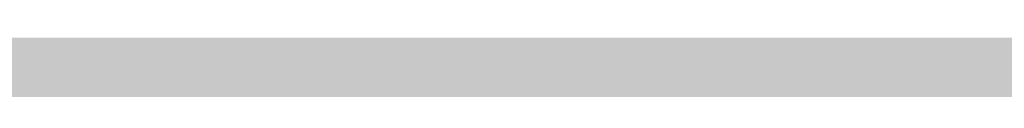
# Model space of a CAD drawing. Units: feet. Extents: x 3168 to 4724, y 827 to 1477.
# Tile 9 of 256: x 3244.72 to 3257.5, y 1098.34 to 1099. Entities that reach past the tile are written whole.
import ezdxf

# ---------------------------------------------------------------- set-up
doc = ezdxf.new("R2010")
doc.units = ezdxf.units.FT
doc.layers.add('A-ELEV', color=7, linetype='Continuous', lineweight=35)
doc.layers.add('A-ELEV-PATT', color=8, linetype='Continuous', lineweight=13)

msp = doc.modelspace()

# ---------------------------------------------------------------- hatches: boundary and pattern name
at = {"layer": 'A-ELEV-PATT'}
h = msp.add_hatch(color=256, dxfattribs=at)
h.dxf.hatch_style = 1
h.paths.add_polyline_path([(3384.525, 1099.016), (3335.029, 1099.016), (3299.317, 1099.016), (3273.143, 1099.016), (3217.565, 1099.016), (3168.069, 827.116), (3335.029, 827.116)])

# ---------------------------------------------------------------- linework, layer by layer
at = {"layer": 'A-ELEV'}
msp.add_open_spline([(3808.52, 1099.016), (3808.52, 1141.413), (3808.52, 1183.81), (3808.52, 1226.635), (3808.52, 1227.064), (3808.52, 1227.492), (3811.492, 1248.995), (3814.464, 1270.498), (3817.465, 1292.218), (3817.495, 1292.435), (3817.525, 1292.652), (3817.573, 1310.107), (3817.62, 1327.562), (3817.668, 1345.016), (3817.668, 1345.458), (3817.668, 1345.9), (3817.668, 1346.456), (3817.668, 1346.571), (3817.668, 1346.753), (3817.668, 1346.82), (3817.668, 1346.935), (3817.668, 1346.982), (3817.668, 1347.039), (3817.668, 1347.047), (3817.668, 1347.074), (3817.668, 1347.059), (3817.668, 1347.062), (3817.668, 1347.063), (3817.668, 1347.066), (3817.668, 1347.068), (3817.668, 1347.075), (3817.668, 1347.079), (3817.668, 1347.093), (3817.668, 1347.102), (3817.668, 1347.129), (3817.668, 1347.147), (3817.667, 1347.2), (3817.667, 1347.236), (3817.666, 1347.343), (3817.665, 1347.415), (3817.661, 1347.628), (3817.657, 1347.77), (3817.64, 1348.192), (3817.624, 1348.472), (3817.559, 1349.3), (3817.496, 1349.841), (3817.255, 1351.424), (3817.026, 1352.429), (3816.307, 1354.889), (3815.744, 1356.269), (3814.464, 1358.819), (3813.746, 1359.991), (3812.196, 1362.172), (3811.362, 1363.182), (3809.589, 1365.069), (3808.649, 1365.946), (3806.654, 1367.58), (3805.6, 1368.336), (3803.353, 1369.722), (3802.161, 1370.352), (3799.601, 1371.454), (3798.233, 1371.925), (3795.28, 1372.635), (3793.693, 1372.872), (3791.869, 1372.926), (3791.741, 1372.929), (3791.353, 1372.934), (3791.093, 1372.933), (3790.304, 1372.915), (3789.77, 1372.884), (3789.209, 1372.83), (3789.191, 1372.828), (3789.135, 1372.823), (3789.098, 1372.819), (3789.048, 1372.814), (3789.036, 1372.813), (3789, 1372.809), (3788.976, 1372.806), (3788.949, 1372.803), (3788.947, 1372.803), (3788.943, 1372.803), (3788.941, 1372.802), (3788.939, 1372.802), (3788.938, 1372.802), (3788.935, 1372.802), (3788.868, 1372.794), (3788.757, 1372.782), (3788.702, 1372.776), (3788.536, 1372.758), (3788.425, 1372.746), (3788.093, 1372.709), (3787.872, 1372.685), (3787.208, 1372.612), (3786.765, 1372.563), (3785.437, 1372.417), (3784.551, 1372.32), (3781.895, 1372.027), (3780.125, 1371.833), (3774.813, 1371.248), (3771.271, 1370.859), (3760.647, 1369.69), (3753.564, 1368.911), (3732.316, 1366.573), (3718.15, 1365.015), (3694.007, 1362.359), (3684.029, 1361.262), (3674.051, 1360.164), (3664.601, 1360.164), (3655.151, 1360.164), (3626.801, 1360.164), (3607.901, 1360.164), (3551.202, 1360.164), (3513.402, 1360.164), (3467.725, 1360.164), (3459.848, 1360.164), (3436.215, 1360.164), (3420.46, 1360.164), (3373.194, 1360.164), (3341.684, 1360.164), (3302.848, 1360.164), (3295.523, 1360.164), (3286.038, 1360.164), (3283.879, 1360.164), (3277.403, 1360.164), (3273.085, 1360.164), (3267.733, 1360.164), (3266.699, 1360.164), (3263.597, 1360.164), (3261.528, 1360.164), (3259.237, 1360.164), (3259.014, 1360.164), (3258.344, 1360.164), (3257.897, 1360.164), (3257.431, 1360.164), (3257.411, 1360.164), (3257.371, 1360.164), (3257.375, 1360.164), (3257.375, 1360.164), (3257.374, 1360.164), (3257.372, 1360.164), (3257.371, 1360.164), (3257.367, 1360.164), (3257.364, 1360.164), (3257.356, 1360.164), (3257.351, 1360.164), (3257.335, 1360.164), (3257.324, 1360.164), (3257.293, 1360.164), (3257.272, 1360.164), (3257.208, 1360.163), (3257.166, 1360.163), (3257.04, 1360.161), (3256.956, 1360.16), (3256.706, 1360.153), (3256.539, 1360.147), (3256.044, 1360.122), (3255.717, 1360.097), (3254.752, 1360), (3254.128, 1359.907), (3252.18, 1359.525), (3250.942, 1359.144), (3248.67, 1358.243), (3247.636, 1357.724), (3245.733, 1356.603), (3244.863, 1356.002), (3243.253, 1354.743), (3242.512, 1354.085), (3240.751, 1352.345), (3239.801, 1351.23), (3238.088, 1348.872), (3237.325, 1347.63), (3235.983, 1344.972), (3235.402, 1343.555), (3234.591, 1340.815), (3234.311, 1339.544), (3233.976, 1336.803), (3233.922, 1335.331), (3234.149, 1332.591), (3234.35, 1331.367), (3234.72, 1329.999), (3234.752, 1329.883), (3234.854, 1329.535), (3234.926, 1329.302), (3235.025, 1329.003), (3235.047, 1328.937), (3235.078, 1328.847), (3235.086, 1328.823), (3235.111, 1328.751), (3235.128, 1328.703), (3235.148, 1328.646), (3235.151, 1328.638), (3235.156, 1328.624), (3235.158, 1328.618), (3235.16, 1328.612), (3235.166, 1328.597), (3235.18, 1328.556), (3235.19, 1328.528), (3235.221, 1328.443), (3235.241, 1328.386), (3235.302, 1328.216), (3235.343, 1328.102), (3235.465, 1327.762), (3235.546, 1327.535), (3235.79, 1326.853), (3235.953, 1326.399), (3236.44, 1325.037), (3236.766, 1324.128), (3237.741, 1321.403), (3238.392, 1319.587), (3240.344, 1314.137), (3241.645, 1310.504), (3245.548, 1299.604), (3248.15, 1292.337), (3255.956, 1270.537), (3261.16, 1256.004), (3267.388, 1238.612), (3268.411, 1235.753), (3269.51, 1232.684), (3269.586, 1232.474), (3269.707, 1232.136), (3269.752, 1232.008), (3269.827, 1231.799), (3269.856, 1231.718), (3269.906, 1231.578), (3269.927, 1231.52), (3269.972, 1231.393), (3269.997, 1231.325), (3270.027, 1231.243), (3270.032, 1231.228), (3270.04, 1231.204), (3270.039, 1231.207), (3270.039, 1231.207), (3270.039, 1231.206), (3270.04, 1231.206), (3270.04, 1231.205), (3270.04, 1231.204), (3270.04, 1231.204), (3270.041, 1231.201), (3270.042, 1231.2), (3270.043, 1231.195), (3270.045, 1231.192), (3270.048, 1231.183), (3270.05, 1231.177), (3270.056, 1231.159), (3270.061, 1231.147), (3270.074, 1231.111), (3270.083, 1231.087), (3270.109, 1231.014), (3270.127, 1230.966), (3270.18, 1230.822), (3270.216, 1230.727), (3270.325, 1230.442), (3270.4, 1230.253), (3270.629, 1229.691), (3270.789, 1229.324), (3271.286, 1228.238), (3271.643, 1227.54), (3272.776, 1225.515), (3273.614, 1224.261), (3275.416, 1221.918), (3276.38, 1220.829), (3278.897, 1218.318), (3280.512, 1216.98), (3283.951, 1214.603), (3285.776, 1213.564), (3289.654, 1211.813), (3291.707, 1211.101), (3294.03, 1210.574), (3294.169, 1210.543), (3294.588, 1210.454), (3294.869, 1210.399), (3295.718, 1210.243), (3296.293, 1210.155), (3296.979, 1210.07), (3297.083, 1210.058), (3297.393, 1210.023), (3297.602, 1210.002), (3298.229, 1209.946), (3298.652, 1209.917), (3299.13, 1209.895), (3299.181, 1209.893), (3299.334, 1209.887), (3299.437, 1209.883), (3299.745, 1209.874), (3299.951, 1209.871), (3300.195, 1209.869), (3300.232, 1209.869), (3300.28, 1209.869), (3300.291, 1209.869), (3300.306, 1209.869), (3300.311, 1209.869), (3300.321, 1209.869), (3300.326, 1209.869), (3300.332, 1209.869), (3300.334, 1209.869), (3300.337, 1209.869), (3300.338, 1209.869), (3300.341, 1209.869), (3300.343, 1209.869), (3300.346, 1209.869), (3300.346, 1209.869), (3300.346, 1209.869), (3300.366, 1209.869), (3300.388, 1209.869), (3300.399, 1209.869), (3300.431, 1209.869), (3300.453, 1209.869), (3300.517, 1209.869), (3300.561, 1209.869), (3300.69, 1209.869), (3300.777, 1209.869), (3301.036, 1209.869), (3301.209, 1209.869), (3301.727, 1209.869), (3302.073, 1209.869), (3303.11, 1209.869), (3303.801, 1209.869), (3305.875, 1209.869), (3307.257, 1209.869), (3311.405, 1209.869), (3314.17, 1209.869), (3322.466, 1209.869), (3327.996, 1209.869), (3344.586, 1209.869), (3355.647, 1209.869), (3388.828, 1209.869), (3410.949, 1209.869), (3477.312, 1209.869), (3521.554, 1209.869), (3566.836, 1209.869), (3567.877, 1209.869), (3570.999, 1209.869), (3573.08, 1209.869), (3575.781, 1209.869), (3576.401, 1209.869), (3577.296, 1209.869), (3577.571, 1209.869), (3578.397, 1209.869), (3578.948, 1209.869), (3579.756, 1209.869), (3580.015, 1209.869), (3580.343, 1209.869), (3580.327, 1209.869), (3580.327, 1209.869), (3580.327, 1209.869), (3580.328, 1209.869), (3580.328, 1209.869), (3580.329, 1209.869), (3580.33, 1209.869), (3580.331, 1209.869), (3580.333, 1209.869), (3580.336, 1209.869), (3580.339, 1209.869), (3580.346, 1209.869), (3580.351, 1209.869), (3580.366, 1209.869), (3580.375, 1209.869), (3580.405, 1209.868), (3580.424, 1209.868), (3580.483, 1209.868), (3580.522, 1209.868), (3580.64, 1209.867), (3580.719, 1209.865), (3580.956, 1209.861), (3581.115, 1209.856), (3581.594, 1209.837), (3581.916, 1209.818), (3582.89, 1209.742), (3583.548, 1209.666), (3585.532, 1209.361), (3586.867, 1209.054), (3589.472, 1208.252), (3590.74, 1207.758), (3591.995, 1207.159), (3592.058, 1207.129), (3592.244, 1207.038), (3592.368, 1206.977), (3592.735, 1206.79), (3592.977, 1206.663), (3593.245, 1206.516), (3593.275, 1206.5), (3593.365, 1206.45), (3593.425, 1206.416), (3593.604, 1206.315), (3593.723, 1206.247), (3593.857, 1206.168), (3593.874, 1206.158), (3593.926, 1206.128), (3593.96, 1206.108), (3594.062, 1206.047), (3594.13, 1206.006), (3594.208, 1205.958), (3594.22, 1205.951), (3594.253, 1205.931), (3594.276, 1205.917), (3594.343, 1205.876), (3594.388, 1205.848), (3594.434, 1205.819), (3594.435, 1205.818), (3594.44, 1205.815), (3594.443, 1205.813), (3594.447, 1205.811), (3594.448, 1205.81), (3594.449, 1205.81), (3594.449, 1205.809), (3594.45, 1205.809), (3594.45, 1205.808), (3594.451, 1205.808), (3594.467, 1205.798), (3594.493, 1205.782), (3594.506, 1205.774), (3594.545, 1205.749), (3594.571, 1205.733), (3594.648, 1205.684), (3594.7, 1205.652), (3594.855, 1205.555), (3594.959, 1205.49), (3595.269, 1205.295), (3595.476, 1205.166), (3596.097, 1204.776), (3596.511, 1204.517), (3597.753, 1203.739), (3598.581, 1203.22), (3601.064, 1201.664), (3602.72, 1200.626), (3607.687, 1197.513), (3610.998, 1195.438), (3620.932, 1189.212), (3627.555, 1185.061), (3647.423, 1172.61), (3660.668, 1164.309), (3700.403, 1139.405), (3726.894, 1122.803), (3757.206, 1103.806), (3761.027, 1101.411), (3764.848, 1099.016), (3745.328, 1099.016), (3725.808, 1099.016), (3706.288, 1099.016), (3706.288, 1108.453), (3706.288, 1117.89), (3706.288, 1127.327), (3710.751, 1127.327), (3715.213, 1127.327), (3719.676, 1127.327)], degree=3, knots=[0, 0, 0, 0, 0.982037, 0.982037, 0.991957, 0.991957, 0.991957, 1.966522, 1.966522, 1.976367, 1.976367, 1.976367, 2.976367, 2.976367, 2.976367, 3.00169, 3.00169, 3.008272, 3.008272, 3.012129, 3.012129, 3.014851, 3.014851, 3.015353, 3.015353, 3.016359, 3.016359, 3.017365, 3.017365, 3.019376, 3.019376, 3.023398, 3.023398, 3.031442, 3.031442, 3.047531, 3.047531, 3.079708, 3.079708, 3.144063, 3.144063, 3.272772, 3.272772, 3.53019, 3.53019, 4.045026, 4.045026, 5.074698, 5.074698, 6.700878, 6.700878, 8.327058, 8.327058, 9.953238, 9.953238, 11.579418, 11.579418, 13.205598, 13.205598, 14.831778, 14.831778, 16.457958, 16.457958, 18.084138, 18.084138, 18.206872, 18.206872, 18.45234, 18.45234, 18.943275, 18.943275, 18.960093, 18.960093, 18.993729, 18.993729, 19.00461, 19.00461, 19.026374, 19.026374, 19.028737, 19.028737, 19.03018, 19.03018, 19.030897, 19.030897, 19.032332, 19.032332, 19.033766, 19.033766, 19.036636, 19.036636, 19.042374, 19.042374, 19.053851, 19.053851, 19.076805, 19.076805, 19.122714, 19.122714, 19.21453, 19.21453, 19.398163, 19.398163, 19.765429, 19.765429, 20.024128, 20.024128, 20.024128, 20.092031, 20.092031, 20.227836, 20.227836, 20.499446, 20.499446, 20.556051, 20.556051, 20.66926, 20.66926, 20.895678, 20.895678, 20.948316, 20.948316, 20.963829, 20.963829, 20.994855, 20.994855, 21.002285, 21.002285, 21.017146, 21.017146, 21.01875, 21.01875, 21.021959, 21.021959, 21.022102, 21.022102, 21.022249, 21.022249, 21.022708, 21.022708, 21.023627, 21.023627, 21.025464, 21.025464, 21.029138, 21.029138, 21.036486, 21.036486, 21.051183, 21.051183, 21.080575, 21.080575, 21.139361, 21.139361, 21.256932, 21.256932, 21.492073, 21.492073, 21.962356, 21.962356, 23.01002, 23.01002, 24.057684, 24.057684, 25.105348, 25.105348, 26.153011, 26.153011, 27.776787, 27.776787, 29.400562, 29.400562, 31.024337, 31.024337, 32.278801, 32.278801, 33.533265, 33.533265, 34.467568, 34.467568, 34.553971, 34.553971, 34.726776, 34.726776, 34.775309, 34.775309, 34.793079, 34.793079, 34.82862, 34.82862, 34.834979, 34.834979, 34.839039, 34.839039, 34.839411, 34.839411, 34.840285, 34.840285, 34.842034, 34.842034, 34.845531, 34.845531, 34.852525, 34.852525, 34.866512, 34.866512, 34.894488, 34.894488, 34.950439, 34.950439, 35.062342, 35.062342, 35.286147, 35.286147, 35.733758, 35.733758, 35.821815, 35.821815, 35.828283, 35.828283, 35.832225, 35.832225, 35.834724, 35.834724, 35.836521, 35.836521, 35.838617, 35.838617, 35.839073, 35.839073, 35.839345, 35.839345, 35.839617, 35.839617, 35.840161, 35.840161, 35.841249, 35.841249, 35.843425, 35.843425, 35.847778, 35.847778, 35.856482, 35.856482, 35.873891, 35.873891, 35.908709, 35.908709, 35.978345, 35.978345, 36.117617, 36.117617, 36.396161, 36.396161, 36.953248, 36.953248, 38.067423, 38.067423, 40.295772, 40.295772, 42.524122, 42.524122, 45.81453, 45.81453, 49.104937, 49.104937, 52.395345, 52.395345, 52.603776, 52.603776, 53.020639, 53.020639, 53.854363, 53.854363, 54.001655, 54.001655, 54.296238, 54.296238, 54.885405, 54.885405, 54.955785, 54.955785, 55.096546, 55.096546, 55.378067, 55.378067, 55.42849, 55.42849, 55.442691, 55.442691, 55.449436, 55.449436, 55.455957, 55.455957, 55.458409, 55.458409, 55.459872, 55.459872, 55.462798, 55.462798, 55.462856, 55.462856, 55.462972, 55.462972, 55.463088, 55.463088, 55.463319, 55.463319, 55.463782, 55.463782, 55.464708, 55.464708, 55.46656, 55.46656, 55.470263, 55.470263, 55.47767, 55.47767, 55.492484, 55.492484, 55.522112, 55.522112, 55.581369, 55.581369, 55.699882, 55.699882, 55.936907, 55.936907, 56.410959, 56.410959, 56.42211, 56.42211, 56.444413, 56.444413, 56.451051, 56.451051, 56.454001, 56.454001, 56.459901, 56.459901, 56.462666, 56.462666, 56.463418, 56.463418, 56.464171, 56.464171, 56.465675, 56.465675, 56.468684, 56.468684, 56.474702, 56.474702, 56.486738, 56.486738, 56.51081, 56.51081, 56.558955, 56.558955, 56.655243, 56.655243, 56.847821, 56.847821, 57.232975, 57.232975, 58.003284, 58.003284, 59.543901, 59.543901, 62.625137, 62.625137, 68.787607, 68.787607, 74.950078, 74.950078, 75.27336, 75.27336, 75.919923, 75.919923, 77.213051, 77.213051, 77.377769, 77.377769, 77.707206, 77.707206, 78.366079, 78.366079, 78.462532, 78.462532, 78.655436, 78.655436, 79.041245, 79.041245, 79.105735, 79.105735, 79.234714, 79.234714, 79.492672, 79.492672, 79.502197, 79.502197, 79.521249, 79.521249, 79.523534, 79.523534, 79.528103, 79.528103, 79.528682, 79.528682, 79.528885, 79.528885, 79.529089, 79.529089, 79.529495, 79.529495, 79.530308, 79.530308, 79.531935, 79.531935, 79.535187, 79.535187, 79.541693, 79.541693, 79.554704, 79.554704, 79.580725, 79.580725, 79.632769, 79.632769, 79.736856, 79.736856, 79.94503, 79.94503, 80.361377, 80.361377, 80.421435, 80.421435, 80.421435, 81.421435, 81.421435, 81.421435, 82.421435, 82.421435, 82.421435, 83.421435, 83.421435, 83.421435, 83.421435], dxfattribs=at)

doc.saveas('drawing.dxf')
